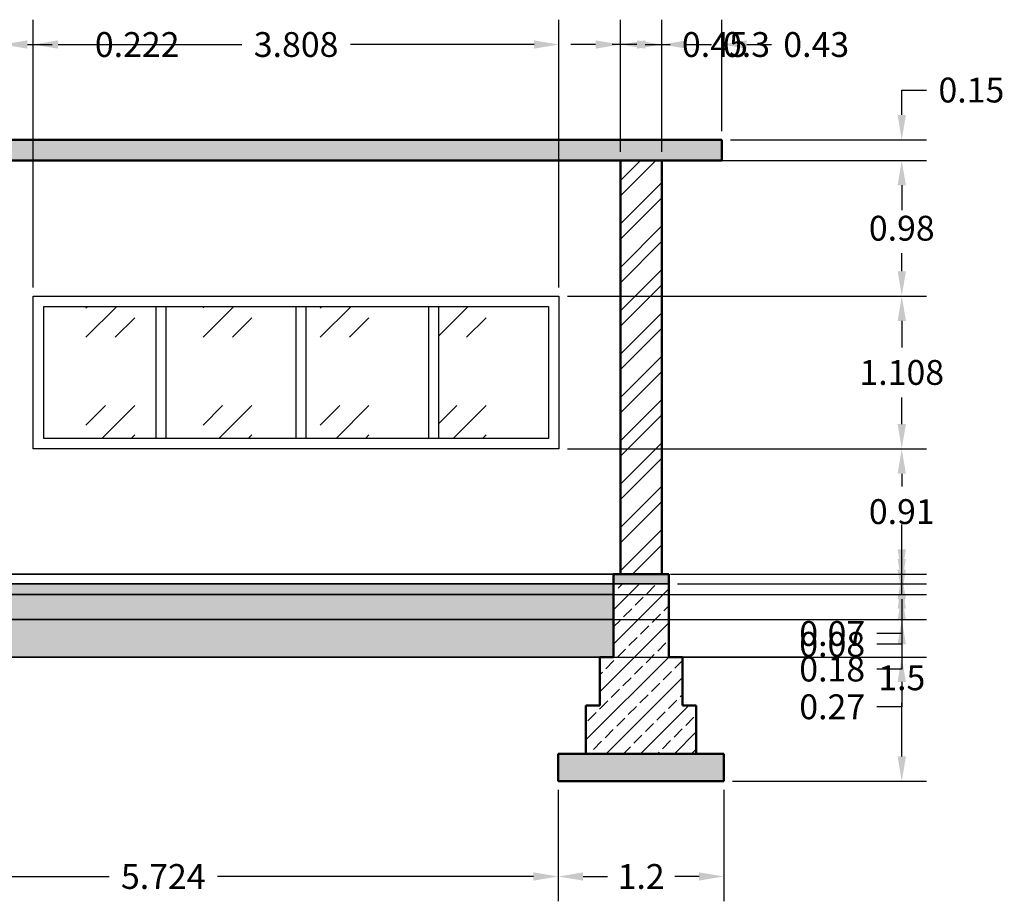
# Model space of a CAD drawing. Units: metres. Extents: x 2294.9 to 2311.3, y 1642.1 to 1648.4.
# Tile 3 of 3: x 2304.1 to 2311.3, y 1642.1 to 1648.4. Entities that reach past the tile are written whole.
import ezdxf

# ---------------------------------------------------------------- set-up
doc = ezdxf.new("R2010")
doc.units = ezdxf.units.M
for name, color, linetype, lineweight in [('A-ANNO-DIMS', 2, 'Continuous', 18), ('A-FLOR', 3, 'Continuous', 35), ('A-FLOR-PATT', 8, 'Continuous', 13), ('A-GLAZ', 4, 'Continuous', 25), ('A-WALL', 7, 'Continuous', 50), ('A-WALL-PATT', 8, 'Continuous', 13), ('C-TOPO', 8, 'Continuous', 35), ('S-FNDN', 1, 'Continuous', 50), ('S-FNDN-PATT', 8, 'Continuous', 13), ('S-SLAB', 1, 'Continuous', 50), ('S-SLAB-PATT', 8, 'Continuous', 13)]:
    doc.layers.add(name, color=color, linetype=linetype, lineweight=lineweight)
doc.styles.get("Standard").update_dxf_attribs({"font": 'arial.ttf'})
doc.dimstyles.get("Standard").update_dxf_attribs({"dimtxt": 0.18, "dimasz": 0.18, "dimexe": 0.18, "dimexo": 0.0625, "dimgap": 0.09, "dimtad": 0, "dimtih": 1, "dimtoh": 1, "dimdec": 4, "dimzin": 0, "dimdsep": 46, "dimtxsty": 'Standard', "dimcen": 0.09, "dimadec": 0, "dimazin": 0, "dimtfac": 1, "dimtdec": 4, "dimtofl": 0, "dimtmove": 0, "dimatfit": 3, "dimfxl": 1, "dimtolj": 1, "dimtzin": 0, "dimarcsym": 0})

# ---------------------------------------------------------------- blocks, each defined once
blk = doc.blocks.new('FOOTING-PCC-PAD')
for p, q in [((1.1996, 0.1999), (-0.0004, 0.1999)), ((-0.0004, 0.1999), (-0.0004, -0.0001)), ((1.1996, -0.0001), (1.1996, 0.1999)), ((-0.0004, -0.0001), (1.1996, -0.0001))]:
    blk.add_line(p, q)
blk = doc.blocks.new('*D12')
at = {"layer": 'A-ANNO-DIMS', "color": 0, "lineweight": -2, "transparency": 16777216}
for p, q in [((2303.0514, 1647.4894), (2303.0514, 1648.4469)), ((2303.9994, 1646.5066), (2303.9994, 1648.4469)), ((2302.8714, 1648.2669), (2302.6914, 1648.2669)), ((2304.1794, 1648.2669), (2304.3594, 1648.2669))]:
    blk.add_line(p, q, dxfattribs=at)
at = {"layer": 'A-ANNO-DIMS', "color": 0, "transparency": 16777216}
for points in [[(2302.8714, 1648.2969), (2302.8714, 1648.2369), (2303.0514, 1648.2669)], [(2304.1794, 1648.2969), (2304.1794, 1648.2369), (2303.9994, 1648.2669)]]:
    blk.add_solid(points, dxfattribs=at)
at = {"layer": 'Defpoints', "color": 0, "transparency": 16777216}
for p in [(2303.9994, 1648.2669), (2303.0514, 1647.4269), (2303.9994, 1646.4441)]:
    blk.add_point(p, dxfattribs=at)
at = {"layer": 'A-ANNO-DIMS', "color": 0, "transparency": 16777216, "insert": (2303.5254, 1648.2669), "char_height": 0.18, "attachment_point": 5}
blk.add_mtext('\\A1;0.948', dxfattribs=at)
blk = doc.blocks.new('*D13')
at = {"layer": 'A-ANNO-DIMS', "color": 0, "lineweight": -2, "transparency": 16777216}
for p, q in [((2303.9994, 1646.5066), (2303.9994, 1648.4469)), ((2304.2214, 1646.5066), (2304.2214, 1648.4469)), ((2303.8194, 1648.2669), (2303.6394, 1648.2669)), ((2304.4014, 1648.2669), (2304.5814, 1648.2669))]:
    blk.add_line(p, q, dxfattribs=at)
at = {"layer": 'A-ANNO-DIMS', "color": 0, "transparency": 16777216}
for points in [[(2303.8194, 1648.2969), (2303.8194, 1648.2369), (2303.9994, 1648.2669)], [(2304.4014, 1648.2969), (2304.4014, 1648.2369), (2304.2214, 1648.2669)]]:
    blk.add_solid(points, dxfattribs=at)
at = {"layer": 'Defpoints', "color": 0, "transparency": 16777216}
for p in [(2304.2214, 1648.2669), (2303.9994, 1646.4441), (2304.2214, 1646.4441)]:
    blk.add_point(p, dxfattribs=at)
at = {"layer": 'A-ANNO-DIMS', "color": 0, "transparency": 16777216, "insert": (2304.9742, 1648.2669), "char_height": 0.18, "attachment_point": 5}
blk.add_mtext('\\A1;0.222', dxfattribs=at)
blk = doc.blocks.new('*D14')
at = {"layer": 'A-ANNO-DIMS', "color": 0, "lineweight": -2, "transparency": 16777216}
for p, q in [((2304.2214, 1646.5066), (2304.2214, 1648.4469)), ((2308.0297, 1646.5066), (2308.0297, 1648.4469)), ((2304.4014, 1648.2669), (2305.7317, 1648.2669)), ((2307.8497, 1648.2669), (2306.5194, 1648.2669))]:
    blk.add_line(p, q, dxfattribs=at)
at = {"layer": 'A-ANNO-DIMS', "color": 0, "transparency": 16777216}
for points in [[(2304.4014, 1648.2969), (2304.4014, 1648.2369), (2304.2214, 1648.2669)], [(2307.8497, 1648.2969), (2307.8497, 1648.2369), (2308.0297, 1648.2669)]]:
    blk.add_solid(points, dxfattribs=at)
at = {"layer": 'Defpoints', "color": 0, "transparency": 16777216}
for p in [(2308.0297, 1648.2669), (2304.2214, 1646.4441), (2308.0297, 1646.4441)]:
    blk.add_point(p, dxfattribs=at)
at = {"layer": 'A-ANNO-DIMS', "color": 0, "transparency": 16777216, "insert": (2306.1256, 1648.2669), "char_height": 0.18, "attachment_point": 5}
blk.add_mtext('\\A1;3.808', dxfattribs=at)
blk = doc.blocks.new('*D15')
at = {"layer": 'A-ANNO-DIMS', "color": 0, "lineweight": -2, "transparency": 16777216}
for p, q in [((2308.0297, 1646.5066), (2308.0297, 1648.4469)), ((2308.4753, 1647.4894), (2308.4753, 1648.4469)), ((2307.8497, 1648.2669), (2307.6697, 1648.2669)), ((2308.6553, 1648.2669), (2308.8353, 1648.2669))]:
    blk.add_line(p, q, dxfattribs=at)
at = {"layer": 'A-ANNO-DIMS', "color": 0, "transparency": 16777216}
for points in [[(2307.8497, 1648.2969), (2307.8497, 1648.2369), (2308.0297, 1648.2669)], [(2308.6553, 1648.2969), (2308.6553, 1648.2369), (2308.4753, 1648.2669)]]:
    blk.add_solid(points, dxfattribs=at)
at = {"layer": 'Defpoints', "color": 0, "transparency": 16777216}
for p in [(2308.4753, 1648.2669), (2308.4753, 1647.4269), (2308.0297, 1646.4441)]:
    blk.add_point(p, dxfattribs=at)
at = {"layer": 'A-ANNO-DIMS', "color": 0, "transparency": 16777216, "insert": (2309.1597, 1648.2669), "char_height": 0.18, "attachment_point": 5}
blk.add_mtext('\\A1;0.45', dxfattribs=at)
blk = doc.blocks.new('*D16')
at = {"layer": 'A-ANNO-DIMS', "color": 0, "lineweight": -2, "transparency": 16777216}
for p, q in [((2308.4753, 1647.4894), (2308.4753, 1648.4469)), ((2308.7753, 1647.4894), (2308.7753, 1648.4469)), ((2308.2953, 1648.2669), (2308.1153, 1648.2669)), ((2308.9553, 1648.2669), (2309.1353, 1648.2669))]:
    blk.add_line(p, q, dxfattribs=at)
at = {"layer": 'A-ANNO-DIMS', "color": 0, "transparency": 16777216}
for points in [[(2308.2953, 1648.2969), (2308.2953, 1648.2369), (2308.4753, 1648.2669)], [(2308.9553, 1648.2969), (2308.9553, 1648.2369), (2308.7753, 1648.2669)]]:
    blk.add_solid(points, dxfattribs=at)
at = {"layer": 'Defpoints', "color": 0, "transparency": 16777216}
for p in [(2308.7753, 1648.2669), (2308.4753, 1647.4269), (2308.7753, 1647.4269)]:
    blk.add_point(p, dxfattribs=at)
at = {"layer": 'A-ANNO-DIMS', "color": 0, "transparency": 16777216, "insert": (2309.3891, 1648.2669), "char_height": 0.18, "attachment_point": 5}
blk.add_mtext('\\A1;0.3', dxfattribs=at)
blk = doc.blocks.new('*D17')
at = {"layer": 'A-ANNO-DIMS', "color": 0, "lineweight": -2, "transparency": 16777216}
for p, q in [((2308.7753, 1647.4894), (2308.7753, 1648.4469)), ((2309.2101, 1647.6394), (2309.2101, 1648.4469)), ((2308.5953, 1648.2669), (2308.4153, 1648.2669)), ((2309.3901, 1648.2669), (2309.5701, 1648.2669))]:
    blk.add_line(p, q, dxfattribs=at)
at = {"layer": 'A-ANNO-DIMS', "color": 0, "transparency": 16777216}
for points in [[(2308.5953, 1648.2969), (2308.5953, 1648.2369), (2308.7753, 1648.2669)], [(2309.3901, 1648.2969), (2309.3901, 1648.2369), (2309.2101, 1648.2669)]]:
    blk.add_solid(points, dxfattribs=at)
at = {"layer": 'Defpoints', "color": 0, "transparency": 16777216}
for p in [(2309.2101, 1648.2669), (2309.2101, 1647.5769), (2308.7753, 1647.4269)]:
    blk.add_point(p, dxfattribs=at)
at = {"layer": 'A-ANNO-DIMS', "color": 0, "transparency": 16777216, "insert": (2309.8939, 1648.2669), "char_height": 0.18, "attachment_point": 5}
blk.add_mtext('\\A1;0.43', dxfattribs=at)
blk = doc.blocks.new('*D21')
at = {"layer": 'A-ANNO-DIMS', "color": 0, "lineweight": -2, "transparency": 16777216}
for p, q in [((2302.3014, 1642.8644), (2302.3014, 1642.0569)), ((2308.0253, 1642.8644), (2308.0253, 1642.0569)), ((2302.4814, 1642.2369), (2304.77, 1642.2369)), ((2307.8453, 1642.2369), (2305.5567, 1642.2369))]:
    blk.add_line(p, q, dxfattribs=at)
at = {"layer": 'A-ANNO-DIMS', "color": 0, "transparency": 16777216}
for points in [[(2302.4814, 1642.2669), (2302.4814, 1642.2069), (2302.3014, 1642.2369)], [(2307.8453, 1642.2669), (2307.8453, 1642.2069), (2308.0253, 1642.2369)]]:
    blk.add_solid(points, dxfattribs=at)
at = {"layer": 'Defpoints', "color": 0, "transparency": 16777216}
for p in [(2302.3014, 1642.9269), (2308.0253, 1642.9269), (2308.0253, 1642.2369)]:
    blk.add_point(p, dxfattribs=at)
at = {"layer": 'A-ANNO-DIMS', "color": 0, "transparency": 16777216, "insert": (2305.1633, 1642.2369), "char_height": 0.18, "attachment_point": 5}
blk.add_mtext('\\A1;5.724', dxfattribs=at)
blk = doc.blocks.new('*D22')
at = {"layer": 'A-ANNO-DIMS', "color": 0, "lineweight": -2, "transparency": 16777216}
for p, q in [((2308.0253, 1642.8644), (2308.0253, 1642.0569)), ((2309.2253, 1642.8644), (2309.2253, 1642.0569)), ((2308.2053, 1642.2369), (2308.3808, 1642.2369)), ((2309.0453, 1642.2369), (2308.8697, 1642.2369))]:
    blk.add_line(p, q, dxfattribs=at)
at = {"layer": 'A-ANNO-DIMS', "color": 0, "transparency": 16777216}
for points in [[(2308.2053, 1642.2669), (2308.2053, 1642.2069), (2308.0253, 1642.2369)], [(2309.0453, 1642.2669), (2309.0453, 1642.2069), (2309.2253, 1642.2369)]]:
    blk.add_solid(points, dxfattribs=at)
at = {"layer": 'Defpoints', "color": 0, "transparency": 16777216}
for p in [(2308.0253, 1642.9269), (2309.2253, 1642.9269), (2309.2253, 1642.2369)]:
    blk.add_point(p, dxfattribs=at)
at = {"layer": 'A-ANNO-DIMS', "color": 0, "transparency": 16777216, "insert": (2308.6253, 1642.2369), "char_height": 0.18, "attachment_point": 5}
blk.add_mtext('\\A1;1.2', dxfattribs=at)
blk = doc.blocks.new('*D35')
at = {"layer": 'A-ANNO-DIMS', "color": 0, "lineweight": -2, "transparency": 16777216}
for p, q in [((2310.5137, 1644.4597), (2310.5137, 1644.6397)), ((2303.1639, 1644.2797), (2310.6937, 1644.2797)), ((2303.1639, 1644.1004), (2310.6937, 1644.1004)), ((2310.5137, 1643.9204), (2310.5137, 1643.7404)), ((2310.5137, 1643.7404), (2310.3337, 1643.7404))]:
    blk.add_line(p, q, dxfattribs=at)
at = {"layer": 'A-ANNO-DIMS', "color": 0, "transparency": 16777216}
for points in [[(2310.4837, 1644.4597), (2310.5437, 1644.4597), (2310.5137, 1644.2797)], [(2310.4837, 1643.9204), (2310.5437, 1643.9204), (2310.5137, 1644.1004)]]:
    blk.add_solid(points, dxfattribs=at)
at = {"layer": 'Defpoints', "color": 0, "transparency": 16777216}
for p in [(2303.1014, 1644.2797), (2303.1014, 1644.1004), (2310.5137, 1644.1004)]:
    blk.add_point(p, dxfattribs=at)
at = {"layer": 'A-ANNO-DIMS', "color": 0, "transparency": 16777216, "insert": (2310.0097, 1643.7404), "char_height": 0.18, "attachment_point": 5}
blk.add_mtext('\\A1;0.18', dxfattribs=at)
blk = doc.blocks.new('*D36')
at = {"layer": 'A-ANNO-DIMS', "color": 0, "lineweight": -2, "transparency": 16777216}
for p, q in [((2310.5137, 1644.2804), (2310.5137, 1644.4604)), ((2303.1639, 1644.1004), (2310.6937, 1644.1004)), ((2303.1639, 1643.8269), (2310.6937, 1643.8269)), ((2310.5137, 1643.6469), (2310.5137, 1643.4669)), ((2310.5137, 1643.4669), (2310.3337, 1643.4669))]:
    blk.add_line(p, q, dxfattribs=at)
at = {"layer": 'A-ANNO-DIMS', "color": 0, "transparency": 16777216}
for points in [[(2310.4837, 1644.2804), (2310.5437, 1644.2804), (2310.5137, 1644.1004)], [(2310.4837, 1643.6469), (2310.5437, 1643.6469), (2310.5137, 1643.8269)]]:
    blk.add_solid(points, dxfattribs=at)
at = {"layer": 'Defpoints', "color": 0, "transparency": 16777216}
for p in [(2303.1014, 1644.1004), (2303.1014, 1643.8269), (2310.5137, 1643.8269)]:
    blk.add_point(p, dxfattribs=at)
at = {"layer": 'A-ANNO-DIMS', "color": 0, "transparency": 16777216, "insert": (2310.0099, 1643.4669), "char_height": 0.18, "attachment_point": 5}
blk.add_mtext('\\A1;0.27', dxfattribs=at)
blk = doc.blocks.new('*D37')
at = {"layer": 'A-ANNO-DIMS', "color": 0, "lineweight": -2, "transparency": 16777216}
for p, q in [((2310.5137, 1644.6069), (2310.5137, 1644.7869)), ((2308.8878, 1644.4269), (2310.6937, 1644.4269)), ((2308.8878, 1644.3583), (2310.6937, 1644.3583)), ((2310.5137, 1644.1783), (2310.5137, 1643.9983)), ((2310.5137, 1643.9983), (2310.3337, 1643.9983))]:
    blk.add_line(p, q, dxfattribs=at)
at = {"layer": 'A-ANNO-DIMS', "color": 0, "transparency": 16777216}
for points in [[(2310.4837, 1644.6069), (2310.5437, 1644.6069), (2310.5137, 1644.4269)], [(2310.4837, 1644.1783), (2310.5437, 1644.1783), (2310.5137, 1644.3583)]]:
    blk.add_solid(points, dxfattribs=at)
at = {"layer": 'Defpoints', "color": 0, "transparency": 16777216}
for p in [(2308.8253, 1644.4269), (2308.8253, 1644.3583), (2310.5137, 1644.3583)]:
    blk.add_point(p, dxfattribs=at)
at = {"layer": 'A-ANNO-DIMS', "color": 0, "transparency": 16777216, "insert": (2310.0099, 1643.9983), "char_height": 0.18, "attachment_point": 5}
blk.add_mtext('\\A1;0.07', dxfattribs=at)
blk = doc.blocks.new('*D38')
at = {"layer": 'A-ANNO-DIMS', "color": 0, "lineweight": -2, "transparency": 16777216}
for p, q in [((2310.5137, 1644.5383), (2310.5137, 1644.7183)), ((2308.8878, 1644.3583), (2310.6937, 1644.3583)), ((2308.4878, 1644.2797), (2310.6937, 1644.2797)), ((2310.5137, 1644.0997), (2310.5137, 1643.9197)), ((2310.5137, 1643.9197), (2310.3337, 1643.9197))]:
    blk.add_line(p, q, dxfattribs=at)
at = {"layer": 'A-ANNO-DIMS', "color": 0, "transparency": 16777216}
for points in [[(2310.4837, 1644.5383), (2310.5437, 1644.5383), (2310.5137, 1644.3583)], [(2310.4837, 1644.0997), (2310.5437, 1644.0997), (2310.5137, 1644.2797)]]:
    blk.add_solid(points, dxfattribs=at)
at = {"layer": 'Defpoints', "color": 0, "transparency": 16777216}
for p in [(2308.8253, 1644.3583), (2308.4253, 1644.2797), (2310.5137, 1644.2797)]:
    blk.add_point(p, dxfattribs=at)
at = {"layer": 'A-ANNO-DIMS', "color": 0, "transparency": 16777216, "insert": (2310.0097, 1643.9197), "char_height": 0.18, "attachment_point": 5}
blk.add_mtext('\\A1;0.08', dxfattribs=at)
blk = doc.blocks.new('*D39')
at = {"layer": 'A-ANNO-DIMS', "color": 0, "lineweight": -2, "transparency": 16777216}
for p, q in [((2310.5137, 1647.7569), (2310.5137, 1647.9369)), ((2310.5137, 1647.9369), (2310.6937, 1647.9369)), ((2309.2726, 1647.5769), (2310.6937, 1647.5769)), ((2309.2726, 1647.4269), (2310.6937, 1647.4269)), ((2310.5137, 1647.2469), (2310.5137, 1647.0669))]:
    blk.add_line(p, q, dxfattribs=at)
at = {"layer": 'A-ANNO-DIMS', "color": 0, "transparency": 16777216}
for points in [[(2310.4837, 1647.7569), (2310.5437, 1647.7569), (2310.5137, 1647.5769)], [(2310.4837, 1647.2469), (2310.5437, 1647.2469), (2310.5137, 1647.4269)]]:
    blk.add_solid(points, dxfattribs=at)
at = {"layer": 'Defpoints', "color": 0, "transparency": 16777216}
for p in [(2309.2101, 1647.5769), (2310.5137, 1647.5769), (2309.2101, 1647.4269)]:
    blk.add_point(p, dxfattribs=at)
at = {"layer": 'A-ANNO-DIMS', "color": 0, "transparency": 16777216, "insert": (2311.0181, 1647.9369), "char_height": 0.18, "attachment_point": 5}
blk.add_mtext('\\A1;0.15', dxfattribs=at)
blk = doc.blocks.new('*D40')
at = {"layer": 'A-ANNO-DIMS', "color": 0, "lineweight": -2, "transparency": 16777216}
for p, q in [((2308.8378, 1647.4269), (2310.6937, 1647.4269)), ((2310.5137, 1647.2469), (2310.5137, 1647.1174)), ((2310.5137, 1646.6241), (2310.5137, 1646.7536)), ((2308.0922, 1646.4441), (2310.6937, 1646.4441))]:
    blk.add_line(p, q, dxfattribs=at)
at = {"layer": 'A-ANNO-DIMS', "color": 0, "transparency": 16777216}
for points in [[(2310.4837, 1647.2469), (2310.5437, 1647.2469), (2310.5137, 1647.4269)], [(2310.4837, 1646.6241), (2310.5437, 1646.6241), (2310.5137, 1646.4441)]]:
    blk.add_solid(points, dxfattribs=at)
at = {"layer": 'Defpoints', "color": 0, "transparency": 16777216}
for p in [(2308.7753, 1647.4269), (2310.5137, 1647.4269), (2308.0297, 1646.4441)]:
    blk.add_point(p, dxfattribs=at)
at = {"layer": 'A-ANNO-DIMS', "color": 0, "transparency": 16777216, "insert": (2310.5137, 1646.9355), "char_height": 0.18, "attachment_point": 5}
blk.add_mtext('\\A1;0.98', dxfattribs=at)
blk = doc.blocks.new('*D41')
at = {"layer": 'A-ANNO-DIMS', "color": 0, "lineweight": -2, "transparency": 16777216}
for p, q in [((2308.0922, 1646.4441), (2310.6937, 1646.4441)), ((2310.5137, 1646.2641), (2310.5137, 1646.072)), ((2310.5137, 1645.5161), (2310.5137, 1645.7082)), ((2308.0922, 1645.3361), (2310.6937, 1645.3361))]:
    blk.add_line(p, q, dxfattribs=at)
at = {"layer": 'A-ANNO-DIMS', "color": 0, "transparency": 16777216}
for points in [[(2310.4837, 1646.2641), (2310.5437, 1646.2641), (2310.5137, 1646.4441)], [(2310.4837, 1645.5161), (2310.5437, 1645.5161), (2310.5137, 1645.3361)]]:
    blk.add_solid(points, dxfattribs=at)
at = {"layer": 'Defpoints', "color": 0, "transparency": 16777216}
for p in [(2308.0297, 1646.4441), (2310.5137, 1646.4441), (2308.0297, 1645.3361)]:
    blk.add_point(p, dxfattribs=at)
at = {"layer": 'A-ANNO-DIMS', "color": 0, "transparency": 16777216, "insert": (2310.5137, 1645.8901), "char_height": 0.18, "attachment_point": 5}
blk.add_mtext('\\A1;1.108', dxfattribs=at)
blk = doc.blocks.new('*D42')
at = {"layer": 'A-ANNO-DIMS', "color": 0, "lineweight": -2, "transparency": 16777216}
for p, q in [((2308.0922, 1645.3361), (2310.6937, 1645.3361)), ((2310.5137, 1645.1561), (2310.5137, 1645.0634)), ((2310.5137, 1644.6069), (2310.5137, 1644.6996)), ((2308.8378, 1644.4269), (2310.6937, 1644.4269))]:
    blk.add_line(p, q, dxfattribs=at)
at = {"layer": 'A-ANNO-DIMS', "color": 0, "transparency": 16777216}
for points in [[(2310.4837, 1645.1561), (2310.5437, 1645.1561), (2310.5137, 1645.3361)], [(2310.4837, 1644.6069), (2310.5437, 1644.6069), (2310.5137, 1644.4269)]]:
    blk.add_solid(points, dxfattribs=at)
at = {"layer": 'Defpoints', "color": 0, "transparency": 16777216}
for p in [(2308.0297, 1645.3361), (2310.5137, 1645.3361), (2308.7753, 1644.4269)]:
    blk.add_point(p, dxfattribs=at)
at = {"layer": 'A-ANNO-DIMS', "color": 0, "transparency": 16777216, "insert": (2310.5137, 1644.8815), "char_height": 0.18, "attachment_point": 5}
blk.add_mtext('\\A1;0.91', dxfattribs=at)
blk = doc.blocks.new('*D43')
at = {"layer": 'A-ANNO-DIMS', "color": 0, "lineweight": -2, "transparency": 16777216}
for p, q in [((2308.8378, 1644.4269), (2310.6937, 1644.4269)), ((2310.5137, 1644.2469), (2310.5137, 1643.8588)), ((2310.5137, 1643.1069), (2310.5137, 1643.495)), ((2309.2878, 1642.9269), (2310.6937, 1642.9269))]:
    blk.add_line(p, q, dxfattribs=at)
at = {"layer": 'A-ANNO-DIMS', "color": 0, "transparency": 16777216}
for points in [[(2310.4837, 1644.2469), (2310.5437, 1644.2469), (2310.5137, 1644.4269)], [(2310.4837, 1643.1069), (2310.5437, 1643.1069), (2310.5137, 1642.9269)]]:
    blk.add_solid(points, dxfattribs=at)
at = {"layer": 'Defpoints', "color": 0, "transparency": 16777216}
for p in [(2308.7753, 1644.4269), (2310.5137, 1644.4269), (2309.2253, 1642.9269)]:
    blk.add_point(p, dxfattribs=at)
at = {"layer": 'A-ANNO-DIMS', "color": 0, "transparency": 16777216, "insert": (2310.5137, 1643.6769), "char_height": 0.18, "attachment_point": 5}
blk.add_mtext('\\A1;1.5', dxfattribs=at)

msp = doc.modelspace()

# ---------------------------------------------------------------- hatches: boundary and pattern name
at = {"layer": 'A-FLOR-PATT'}
h = msp.add_hatch(dxfattribs=at)
h.set_pattern_fill('JIS_STN_2.5', color=256, scale=0.07)
h.paths.add_polyline_path([(2297.3746, 1644.3583), (2296.9746, 1644.3583), (2296.9746, 1644.3269), (2296.9746, 1643.8269), (2296.8746, 1643.8269), (2296.8746, 1643.4769), (2296.7746, 1643.4769), (2296.7746, 1643.1269), (2297.5746, 1643.1269), (2297.5746, 1643.4769), (2297.4746, 1643.4769), (2297.4746, 1643.8269), (2297.3746, 1643.8269)])
h.paths.add_polyline_path([(2300.0343, 1643.8269), (2299.9412, 1643.8269), (2299.9412, 1644.3583), (2299.5412, 1644.3583), (2299.5412, 1643.8269), (2299.4343, 1643.8269), (2299.4343, 1643.4769), (2299.6329, 1643.4769), (2299.6744, 1643.5859), (2299.6809, 1643.3504), (2299.7223, 1643.4769), (2300.0343, 1643.4769)])
h.paths.add_polyline_path([(2303.2014, 1643.8269), (2303.1014, 1643.8269), (2303.1014, 1644.3583), (2302.7014, 1644.3583), (2302.7014, 1643.8269), (2302.6014, 1643.8269), (2302.6014, 1643.4769), (2302.5014, 1643.4769), (2302.5014, 1643.1269), (2303.3014, 1643.1269), (2303.3014, 1643.4769), (2303.2014, 1643.4769)])
h.paths.add_polyline_path([(2308.9253, 1643.8269), (2308.8253, 1643.8269), (2308.8253, 1644.3583), (2308.4253, 1644.3583), (2308.4253, 1643.8269), (2308.3253, 1643.8269), (2308.3253, 1643.4769), (2308.2253, 1643.4769), (2308.2253, 1643.1269), (2309.0253, 1643.1269), (2309.0253, 1643.4769), (2308.9253, 1643.4769)])
h = msp.add_hatch(dxfattribs=at)
h.set_pattern_fill('AR-SAND', color=256, scale=0.001)
h.paths.add_polyline_path([(2302.7014, 1644.3583), (2299.9412, 1644.3583), (2299.9412, 1644.2797), (2302.7014, 1644.2797)])
h.paths.add_polyline_path([(2308.4253, 1644.3583), (2303.1014, 1644.3583), (2303.1014, 1644.2797), (2308.4253, 1644.2797)])
h = msp.add_hatch(dxfattribs=at)
h.set_pattern_fill('AR-CONC', color=256, scale=0.002)
h.paths.add_polyline_path([(2299.5412, 1644.2797), (2297.3746, 1644.2797), (2297.3746, 1644.1004), (2299.5412, 1644.1004)])
h.paths.add_polyline_path([(2302.7014, 1644.2797), (2299.9412, 1644.2797), (2299.9412, 1644.1004), (2302.7014, 1644.1004)])
h.paths.add_polyline_path([(2308.4253, 1644.2797), (2303.1014, 1644.2797), (2303.1014, 1644.1004), (2308.4253, 1644.1004)])
h = msp.add_hatch(dxfattribs=at)
h.set_pattern_fill('GRAVEL', color=256, scale=0.01)
h.set_pattern_definition([(228.0127875, (0.18288, 0.254), (-2.03200000016, -2.28599999986), [0.034172144, -3.383048364]), (184.969741, (0.16002, 0.2286), (3.047999998794, 0.25400001447), [0.058640472, -5.80540489]), (132.5104471, (0.1016, 0.22352), (2.54000000107, -2.793999999025), [0.041348152, -4.09347228]), (267.273689, (0.00254, 0.16002), (0.25400000053, 5.079999999973), [0.053400452, -5.286643743]), (292.8336542, (0, 0.10668), (-1.270000000106, 3.047999999956), [0.05236337, -5.183980775]), (357.273689, (0.02032, 0.05842), (-5.079999999973, 0.25400000053), [0.053400452, -5.286643743]), (37.69424047, (0.07366, 0.05588), (-3.301999999854, -2.54000000019), [0.070619366, -6.991311531]), (72.25532837, (0.12954, 0.09906), (1.778000000478, 5.587999999848), [0.066671952, -6.60052566]), (121.4295656, (0.14986, 0.16256), (-2.03200000029, 3.301999999823), [0.0535813, -5.30455457]), (175.2363583, (0.12192, 0.20828), (2.79399999996, -0.25400000044), [0.061171328, -2.997393695]), (222.3974378, (0.06096, 0.21336), (-3.047999999902, -2.794000000106), [0.079107792, -7.831677251]), (138.8140748, (0.254, 0.15748), (-1.7779999999, 1.52400000012), [0.027000454, -2.673056582]), (171.4692344, (0.23368, 0.17526), (3.30200000009, -0.507999999424), [0.051368198, -5.0854639]), (225, (0.18288, 0.18288), (0, -0.254), [0.035920934, -0.32328931]), (203.1985905, (0.1651, 0.21336), (1.27000000003, 0.5079999999), [0.019344132, -1.915062237]), (291.8014095, (0.14732, 0.20574), (-0.25400000005, 0.762), [0.027356562, -1.3404753]), (30.9637565, (0.15748, 0.18034), (0.762, 0.508), [0.044431966, -1.436629815]), (161.5650512, (0.19558, 0.2032), (0.508, -0.254), [0.032128714, -0.771089812]), (16.38954033, (0, 0.20574), (2.54, 0.762), [0.0450088, -4.455882667]), (70.34617594, (0.04318, 0.21844), (-1.01600000009, -2.79399999997), [0.037759894, -3.738221568]), (293.1985905, (0.19558, 0.254), (-0.5079999999, 1.27000000004), [0.03868801, -1.89571836]), (343.61045967, (0.21082, 0.21844), (-2.54000000005, 0.76199999982), [0.0450088, -4.455882667]), (339.4439548, (0, 0.04826), (-1.27, 0.508), [0.04340352, -2.126773431]), (294.7751406, (0.04064, 0.03302), (-1.27000000151, 2.79399999931), [0.036367212, -3.600359338]), (66.8014095, (0.19812, 0), (0.50799999992, 1.27000000003), [0.03868801, -1.89571836]), (17.35402464, (0.21336, 0.03556), (-3.301999999934, -1.01600000021), [0.042578274, -4.215237598]), (69.4439548, (0.07366, 0), (-0.508, -1.27), [0.02170176, -2.148475191]), (101.3099325, (0.18288, 0), (-0.254, 1.016), [0.01295146, -1.282199496]), (165.9637565, (0.18034, 0.0127), (0.762, -0.254), [0.05236337, -0.99490546]), (186.00900596, (0.12954, 0.0254), (2.539999999987, 0.25400000013), [0.0485267, -4.804136486]), (303.6900675, (0.15748, 0.15748), (-0.254, 0.508), [0.036632388, -0.879177636]), (353.1572266, (0.1778, 0.127), (4.318000000027, -0.507999999774), [0.063955676, -6.331600907]), (60.9453959, (0.2413, 0.11938), (-1.01600000003, -1.77799999998), [0.026150824, -2.588939232]), (90, (0.254, 0.14224), (-0.254, 0.254), [0.01524, -0.23876]), (120.25643716, (0.12446, 0.03302), (1.01599999988, -1.77800000007), [0.035286696, -3.493394077]), (48.0127875, (0.10668, 0.0635), (2.03200000017, 2.28599999985), [0.068344288, -3.34887622]), (0, (0.1524, 0.1143), (0.254, 0.254), [0.06604, -0.18796]), (325.3048465, (0.21844, 0.1143), (2.54000000096, -1.77799999863), [0.040160956, -3.975931672]), (254.0546041, (0.25146, 0.09144), (-0.254, -1.016), [0.036982908, -1.812165004]), (207.64597536, (0.2413, 0.05588), (-4.826000000177, -2.539999999663), [0.06021451, -5.961246442]), (175.42607874, (0.18796, 0.02794), (-3.302, 0.254), [0.063702946, -6.306584646])])
h.paths.add_polyline_path([(2299.5412, 1644.1004), (2297.3746, 1644.1004), (2297.3746, 1643.8269), (2297.4746, 1643.8269), (2299.5412, 1643.8269)])
h.paths.add_polyline_path([(2302.7014, 1644.1004), (2299.9412, 1644.1004), (2299.9412, 1643.8269), (2302.7014, 1643.8269)])
h.paths.add_polyline_path([(2308.4253, 1644.1004), (2303.1014, 1644.1004), (2303.1014, 1643.8269), (2308.4253, 1643.8269)])
at = {"layer": 'A-GLAZ'}
h = msp.add_hatch(dxfattribs=at)
h.set_pattern_fill('GOST_GLASS', color=256, scale=0.1)
h.paths.add_polyline_path([(2305.1109, 1646.3685), (2304.2971, 1646.3685), (2304.2971, 1645.4118), (2305.1109, 1645.4118)])
h.paths.add_polyline_path([(2306.1256, 1646.3685), (2305.185, 1646.3685), (2305.185, 1645.4118), (2306.1256, 1645.4118)])
h.paths.add_polyline_path([(2307.0861, 1646.3685), (2306.1987, 1646.3685), (2306.1987, 1645.4118), (2307.0861, 1645.4118)])
h.paths.add_polyline_path([(2307.954, 1646.3685), (2307.1593, 1646.3685), (2307.1593, 1645.4118), (2307.954, 1645.4118)])
at = {"layer": 'A-WALL-PATT'}
h = msp.add_hatch(dxfattribs=at)
h.set_pattern_fill('STEEL', color=256, scale=0.07)
h.set_pattern_definition([(45, (0, 0), (-0.157154482, 0.157154482), []), (45, (0, 0.11113), (-0.157154482, 0.157154482), [])])
h.paths.add_polyline_path([(2308.7753, 1647.4269), (2308.4753, 1647.4269), (2308.4753, 1644.4269), (2308.7753, 1644.4269)])
at = {"layer": 'S-FNDN-PATT'}
h = msp.add_hatch(dxfattribs=at)
h.set_pattern_fill('AR-CONC', color=256, scale=0.001)
h.paths.add_polyline_path([(2297.7746, 1643.1269), (2296.5746, 1643.1269), (2296.5746, 1642.9269), (2297.7746, 1642.9269)])
h.paths.add_polyline_path([(2303.5014, 1643.1269), (2302.3014, 1643.1269), (2302.3014, 1642.9269), (2303.5014, 1642.9269)])
h.paths.add_polyline_path([(2309.2253, 1643.1269), (2308.0253, 1643.1269), (2308.0253, 1642.9269), (2309.2253, 1642.9269)])
h.paths.add_polyline_path([(2297.3746, 1644.4269), (2297.3246, 1644.4269), (2297.0246, 1644.4269), (2296.9746, 1644.4269), (2296.9746, 1644.3583), (2297.3746, 1644.3583)])
h.paths.add_polyline_path([(2299.9412, 1644.4269), (2299.7412, 1644.4269), (2299.5412, 1644.4269), (2299.5412, 1644.3583), (2299.9412, 1644.3583)])
h.paths.add_polyline_path([(2303.1014, 1644.4269), (2303.0514, 1644.4269), (2302.7514, 1644.4269), (2302.7014, 1644.4269), (2302.7014, 1644.3583), (2303.1014, 1644.3583)])
h.paths.add_polyline_path([(2308.8253, 1644.4269), (2308.7753, 1644.4269), (2308.4753, 1644.4269), (2308.4253, 1644.4269), (2308.4253, 1644.3583), (2308.8253, 1644.3583)])
at = {"layer": 'S-SLAB-PATT'}
h = msp.add_hatch(dxfattribs=at)
h.set_pattern_fill('AR-CONC', color=256, scale=0.002)
h.paths.add_polyline_path([(2309.2101, 1647.5769), (2296.8101, 1647.5769), (2296.8101, 1647.4269), (2297.1746, 1647.4269), (2308.6282, 1647.4269), (2309.2101, 1647.4269)])

# ---------------------------------------------------------------- linework, layer by layer
at = {"layer": 'A-FLOR'}
for p, q in [((2303.0514, 1644.4269), (2308.4253, 1644.4269)), ((2296.9746, 1644.3583), (2308.8253, 1644.3583)), ((2303.1014, 1644.2797), (2308.4253, 1644.2797)), ((2303.1014, 1644.1004), (2308.4253, 1644.1004)), ((2303.1014, 1643.8269), (2308.4253, 1643.8269))]:
    msp.add_line(p, q, dxfattribs=at)
at = {"layer": 'A-GLAZ'}
for p, q in [((2305.1109, 1645.4118), (2305.1109, 1646.3685)), ((2305.185, 1645.4118), (2305.185, 1646.3685)), ((2306.1256, 1645.4118), (2306.1256, 1646.3685)), ((2306.1987, 1645.4118), (2306.1987, 1646.3685)), ((2307.0861, 1645.4118), (2307.0861, 1646.3685)), ((2307.1593, 1645.4118), (2307.1593, 1646.3685))]:
    msp.add_line(p, q, dxfattribs=at)
for points in [[(2304.2214, 1646.4441), (2308.0297, 1646.4441), (2308.0297, 1645.3361), (2304.2214, 1645.3361)], [(2304.2971, 1646.3685), (2307.954, 1646.3685), (2307.954, 1645.4118), (2304.2971, 1645.4118)]]:
    msp.add_lwpolyline(points, close=True, dxfattribs=at)
at = {"layer": 'A-WALL'}
for p, q in [((2308.4753, 1644.4269), (2308.4753, 1647.4269)), ((2308.7753, 1644.4269), (2308.7753, 1647.4269)), ((2308.4753, 1644.4269), (2308.7753, 1644.4269))]:
    msp.add_line(p, q, dxfattribs=at)
at = {"layer": 'C-TOPO'}
msp.add_line((2308.8253, 1643.8269), (2309.8237, 1643.8269), dxfattribs=at)
at = {"layer": 'S-FNDN'}
for p, q in [((2308.4253, 1643.8269), (2308.4253, 1644.4269)), ((2308.4253, 1644.4269), (2308.4753, 1644.4269)), ((2308.7753, 1644.4269), (2308.8253, 1644.4269)), ((2308.8253, 1644.4269), (2308.8253, 1643.8269)), ((2308.3253, 1643.4769), (2308.3253, 1643.8269)), ((2308.3253, 1643.8269), (2308.4253, 1643.8269)), ((2308.8253, 1643.8269), (2308.9253, 1643.8269)), ((2308.9253, 1643.8269), (2308.9253, 1643.4769)), ((2308.2253, 1643.1269), (2308.2253, 1643.4769)), ((2308.2253, 1643.4769), (2308.3253, 1643.4769)), ((2308.9253, 1643.4769), (2309.0253, 1643.4769)), ((2309.0253, 1643.4769), (2309.0253, 1643.1269))]:
    msp.add_line(p, q, dxfattribs=at)
at = {"layer": 'S-SLAB'}
for p, q in [((2296.8101, 1647.5769), (2309.2101, 1647.5769)), ((2309.2101, 1647.5769), (2309.2101, 1647.4269)), ((2297.1746, 1647.4269), (2308.6282, 1647.4269)), ((2309.2101, 1647.4269), (2297.3246, 1647.4269))]:
    msp.add_line(p, q, dxfattribs=at)

# ---------------------------------------------------------------- block references
at = {"layer": 'S-FNDN'}
msp.add_blockref('FOOTING-PCC-PAD', (2308.0257, 1642.927), dxfattribs=at)

# ---------------------------------------------------------------- dimensions: what is measured, and where the dimension line sits
at = {"layer": 'A-ANNO-DIMS'}
for base, p1, p2, override, picture, middle in [((2303.9994, 1648.2669), (2303.0514, 1647.4269), (2303.9994, 1646.4441), {"dimdec": 3, "dimlfac": 1, "dimrnd": 0, "dimzin": 0, "dimdsep": 46, "dimlunit": 2}, '*D12', (2303.5254, 1648.2669)), ((2304.2214, 1648.2669), (2303.9994, 1646.4441), (2304.2214, 1646.4441), {"dimdec": 3, "dimlfac": 1, "dimrnd": 0, "dimzin": 0, "dimdsep": 46, "dimlunit": 2}, '*D13', (2304.9742, 1648.2669)), ((2308.0297, 1648.2669), (2304.2214, 1646.4441), (2308.0297, 1646.4441), {"dimdec": 3, "dimlfac": 1, "dimrnd": 0, "dimzin": 0, "dimdsep": 46, "dimlunit": 2}, '*D14', (2306.1256, 1648.2669)), ((2308.4753, 1648.2669), (2308.0297, 1646.4441), (2308.4753, 1647.4269), {"dimdec": 2, "dimlfac": 1, "dimrnd": 0, "dimzin": 0, "dimdsep": 46, "dimlunit": 2}, '*D15', (2309.1597, 1648.2669)), ((2308.7753, 1648.2669), (2308.4753, 1647.4269), (2308.7753, 1647.4269), {"dimdec": 1, "dimlfac": 1, "dimrnd": 0, "dimzin": 0, "dimdsep": 46, "dimlunit": 2}, '*D16', (2309.3891, 1648.2669)), ((2309.2101, 1648.2669), (2308.7753, 1647.4269), (2309.2101, 1647.5769), {"dimdec": 2, "dimlfac": 1, "dimrnd": 0, "dimzin": 0, "dimdsep": 46, "dimlunit": 2}, '*D17', (2309.8939, 1648.2669)), ((2308.0253, 1642.2369), (2302.3014, 1642.9269), (2308.0253, 1642.9269), {"dimdec": 3, "dimlfac": 1, "dimrnd": 0, "dimzin": 0, "dimdsep": 46, "dimlunit": 2}, '*D21', (2305.1633, 1642.2369)), ((2309.2253, 1642.2369), (2308.0253, 1642.9269), (2309.2253, 1642.9269), {"dimdec": 1, "dimlfac": 1, "dimrnd": 0, "dimzin": 0, "dimdsep": 46, "dimlunit": 2}, '*D22', (2308.6253, 1642.2369))]:
    dim = msp.add_linear_dim(base=base, p1=p1, p2=p2, dimstyle='Standard', override=override, dxfattribs=at)
    dim.commit()
    dim.dimension.update_dxf_attribs({"geometry": picture, "text_midpoint": middle})
for base, p1, p2, override, picture, middle in [((2310.5137, 1647.5769), (2309.2101, 1647.4269), (2309.2101, 1647.5769), {"dimdec": 2, "dimlfac": 1, "dimrnd": 0, "dimzin": 0, "dimdsep": 46, "dimlunit": 2}, '*D39', (2311.0181, 1647.9369)), ((2310.5137, 1647.4269), (2308.0297, 1646.4441), (2308.7753, 1647.4269), {"dimdec": 2, "dimlfac": 1, "dimrnd": 0, "dimzin": 0, "dimdsep": 46, "dimlunit": 2}, '*D40', (2310.5137, 1646.9355)), ((2310.5137, 1646.4441), (2308.0297, 1645.3361), (2308.0297, 1646.4441), {"dimdec": 3, "dimlfac": 1, "dimrnd": 0, "dimzin": 0, "dimdsep": 46, "dimlunit": 2}, '*D41', (2310.5137, 1645.8901)), ((2310.5137, 1645.3361), (2308.7753, 1644.4269), (2308.0297, 1645.3361), {"dimdec": 2, "dimlfac": 1, "dimrnd": 0, "dimzin": 0, "dimdsep": 46, "dimlunit": 2}, '*D42', (2310.5137, 1644.8815)), ((2310.5137, 1644.3583), (2308.8253, 1644.4269), (2308.8253, 1644.3583), {"dimdec": 2, "dimlfac": 1, "dimrnd": 0, "dimzin": 0, "dimdsep": 46, "dimlunit": 2}, '*D37', (2310.0099, 1643.9983)), ((2310.5137, 1644.2797), (2308.8253, 1644.3583), (2308.4253, 1644.2797), {"dimdec": 2, "dimlfac": 1, "dimrnd": 0, "dimzin": 0, "dimdsep": 46, "dimlunit": 2}, '*D38', (2310.0097, 1643.9197)), ((2310.5137, 1644.1004), (2303.1014, 1644.2797), (2303.1014, 1644.1004), {"dimdec": 2, "dimlfac": 1, "dimrnd": 0, "dimzin": 0, "dimdsep": 46, "dimlunit": 2}, '*D35', (2310.0097, 1643.7404)), ((2310.5137, 1643.8269), (2303.1014, 1644.1004), (2303.1014, 1643.8269), {"dimdec": 2, "dimlfac": 1, "dimrnd": 0, "dimzin": 0, "dimdsep": 46, "dimlunit": 2}, '*D36', (2310.0099, 1643.4669)), ((2310.5137, 1644.4269), (2309.2253, 1642.9269), (2308.7753, 1644.4269), {"dimdec": 1, "dimlfac": 1, "dimrnd": 0, "dimzin": 0, "dimdsep": 46, "dimlunit": 2}, '*D43', (2310.5137, 1643.6769))]:
    dim = msp.add_linear_dim(base=base, p1=p1, p2=p2, angle=90, dimstyle='Standard', override=override, dxfattribs=at)
    dim.commit()
    dim.dimension.update_dxf_attribs({"geometry": picture, "text_midpoint": middle})

doc.saveas('drawing.dxf')
